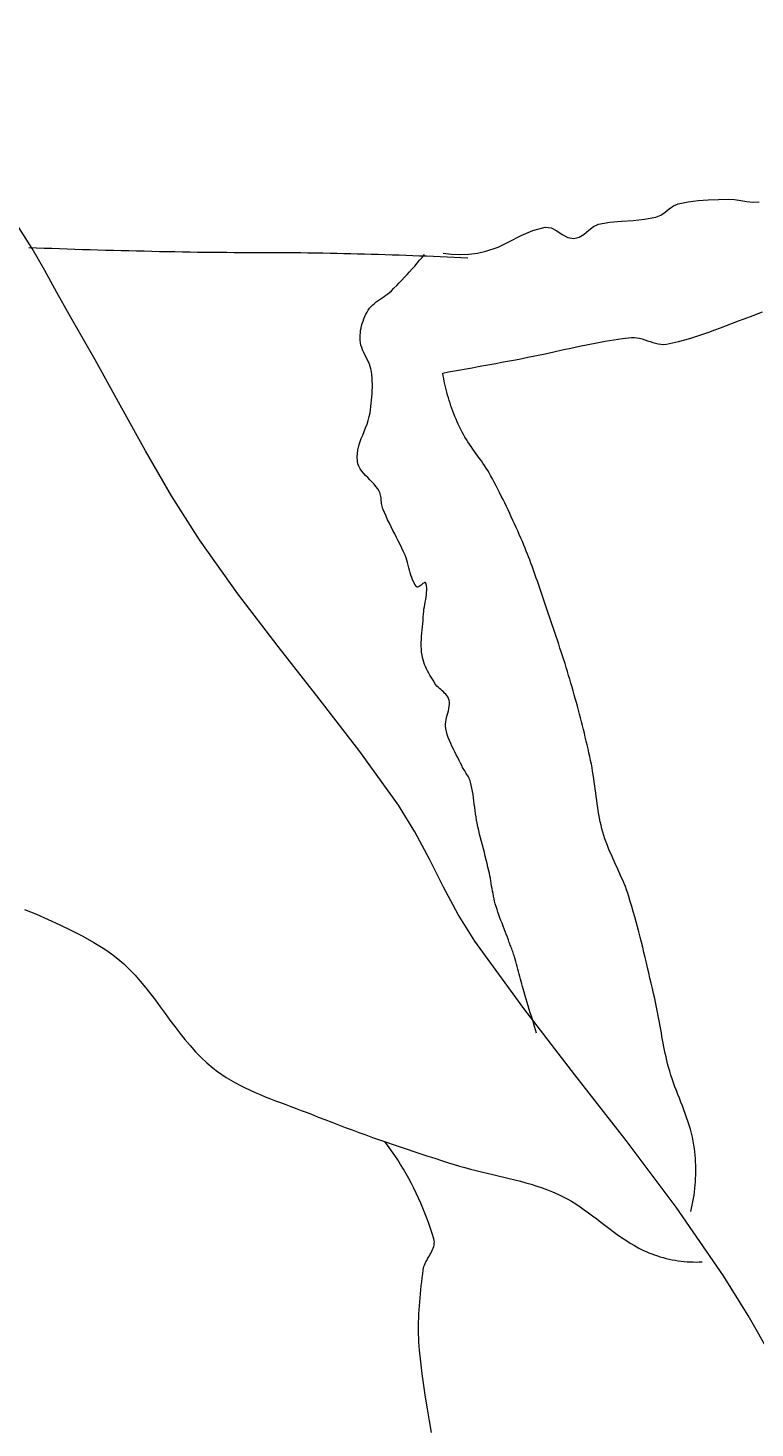
# Model space of a CAD drawing. Units: inches. Extents: x 1441 to 2460, y 1648 to 2683.
# Tile 17 of 35: x 1845 to 1861, y 2091 to 2122. Entities that reach past the tile are written whole.
import ezdxf

# ---------------------------------------------------------------- set-up
doc = ezdxf.new("R2010")
doc.units = ezdxf.units.IN
doc.layers.add('A-ANNO-DIMS', color=2, linetype='Continuous', lineweight=18)
doc.layers.add('A-FURN', color=8, linetype='Continuous', lineweight=15)
doc.styles.get("Standard").update_dxf_attribs({"font": 'arial.ttf'})
doc.dimstyles.get("Standard").update_dxf_attribs({"dimtxt": 0.18, "dimasz": 0.18, "dimexe": 0.18, "dimexo": 0.0625, "dimgap": 0.09, "dimtad": 0, "dimtih": 1, "dimtoh": 1, "dimdec": 4, "dimzin": 0, "dimdsep": 46, "dimtxsty": 'Standard', "dimcen": 0.09, "dimadec": 0, "dimazin": 0, "dimtfac": 1, "dimtdec": 4, "dimtofl": 0, "dimtmove": 0, "dimatfit": 3, "dimfxl": 1, "dimtolj": 1, "dimtzin": 0, "dimarcsym": 0})

# ---------------------------------------------------------------- blocks, each defined once
blk = doc.blocks.new('BED-DOUBLE-PLAN')
for p, q in [((7.216, 72.957), (7.14, 73.155)), ((30.052, 73.35), (29.164, 72.842)), ((4.72, 72.818), (4.732, 72.953)), ((4.732, 72.953), (4.722, 73.087)), ((7.289, 72.758), (7.216, 72.957)), ((29.164, 72.842), (28.298, 72.301)), ((4.668, 72.41), (4.675, 72.546)), ((4.675, 72.546), (4.697, 72.682)), ((4.697, 72.682), (4.72, 72.818)), ((7.337, 72.628), (7.289, 72.758)), ((7.386, 72.498), (7.337, 72.628)), ((4.673, 72.189), (4.668, 72.41)), ((7.436, 72.369), (7.386, 72.498)), ((7.486, 72.239), (7.436, 72.369)), ((7.535, 72.109), (7.486, 72.239)), ((28.298, 72.301), (26.791, 71.264)), ((4.68, 71.967), (4.673, 72.189)), ((4.695, 71.746), (4.68, 71.967)), ((7.583, 71.979), (7.535, 72.109)), ((7.63, 71.848), (7.583, 71.979)), ((4.722, 71.527), (4.695, 71.746)), ((7.675, 71.717), (7.63, 71.848)), ((7.717, 71.585), (7.675, 71.717)), ((25.162, 71.599), (25.076, 71.576)), ((25.25, 71.62), (25.162, 71.599)), ((25.337, 71.638), (25.25, 71.62)), ((25.426, 71.654), (25.337, 71.638)), ((25.498, 71.664), (25.426, 71.654)), ((25.571, 71.673), (25.498, 71.664)), ((25.644, 71.68), (25.571, 71.673)), ((25.717, 71.686), (25.644, 71.68)), ((25.79, 71.691), (25.717, 71.686)), ((25.864, 71.694), (25.79, 71.691)), ((25.938, 71.695), (25.864, 71.694)), ((26.011, 71.695), (25.938, 71.695)), ((26.085, 71.694), (26.011, 71.695)), ((26.159, 71.691), (26.085, 71.694)), ((26.233, 71.687), (26.159, 71.691)), ((26.306, 71.681), (26.233, 71.687)), ((26.379, 71.674), (26.306, 71.681)), ((26.453, 71.665), (26.379, 71.674)), ((26.525, 71.655), (26.453, 71.665)), ((26.598, 71.643), (26.525, 71.655)), ((26.67, 71.63), (26.598, 71.643)), ((26.742, 71.616), (26.67, 71.63)), ((26.814, 71.6), (26.742, 71.616)), ((26.885, 71.583), (26.814, 71.6)), ((27.992, 71.766), (27.99, 71.832)), ((27.99, 71.568), (27.992, 71.634)), ((27.993, 71.7), (27.992, 71.766)), ((27.992, 71.634), (27.993, 71.7)), ((4.765, 71.311), (4.722, 71.527)), ((4.809, 71.206), (4.765, 71.311)), ((7.755, 71.452), (7.717, 71.585)), ((7.79, 71.318), (7.755, 71.452)), ((7.821, 71.184), (7.79, 71.318)), ((24.313, 71.301), (24.228, 71.268)), ((24.397, 71.334), (24.313, 71.301)), ((24.481, 71.366), (24.397, 71.334)), ((24.566, 71.399), (24.481, 71.366)), ((24.65, 71.431), (24.566, 71.399)), ((24.735, 71.463), (24.65, 71.431)), ((24.819, 71.493), (24.735, 71.463)), ((24.904, 71.523), (24.819, 71.493)), ((24.99, 71.55), (24.904, 71.523)), ((25.076, 71.576), (24.99, 71.55)), ((27.953, 71.239), (27.964, 71.304)), ((27.964, 71.304), (27.972, 71.37)), ((27.972, 71.37), (27.98, 71.436)), ((27.98, 71.436), (27.985, 71.502)), ((27.985, 71.502), (27.99, 71.568)), ((4.876, 71.111), (4.809, 71.206)), ((4.95, 71.019), (4.876, 71.111)), ((5.017, 70.924), (4.95, 71.019)), ((7.846, 71.048), (7.821, 71.184)), ((7.852, 70.989), (7.846, 71.048)), ((7.85, 70.93), (7.852, 70.989)), ((23.192, 70.98), (23.116, 70.966)), ((23.267, 70.995), (23.192, 70.98)), ((23.342, 71.01), (23.267, 70.995)), ((23.417, 71.025), (23.342, 71.01)), ((23.492, 71.042), (23.417, 71.025)), ((23.567, 71.059), (23.492, 71.042)), ((23.641, 71.077), (23.567, 71.059)), ((23.715, 71.097), (23.641, 71.077)), ((23.802, 71.121), (23.715, 71.097)), ((23.888, 71.147), (23.802, 71.121)), ((23.974, 71.176), (23.888, 71.147)), ((24.059, 71.205), (23.974, 71.176)), ((24.144, 71.236), (24.059, 71.205)), ((24.228, 71.268), (24.144, 71.236)), ((26.791, 71.264), (25.327, 70.164)), ((27.877, 70.915), (27.895, 70.979)), ((27.895, 70.979), (27.912, 71.044)), ((27.912, 71.044), (27.927, 71.108)), ((27.927, 71.108), (27.941, 71.173)), ((27.941, 71.173), (27.953, 71.239)), ((5.062, 70.82), (5.017, 70.924)), ((5.108, 70.571), (5.062, 70.82)), ((7.772, 70.636), (7.792, 70.694)), ((7.792, 70.694), (7.811, 70.753)), ((7.811, 70.753), (7.828, 70.812)), ((7.828, 70.812), (7.842, 70.871)), ((7.842, 70.871), (7.85, 70.93)), ((21.761, 70.689), (21.648, 70.663)), ((21.874, 70.715), (21.761, 70.689)), ((21.987, 70.741), (21.874, 70.715)), ((22.1, 70.767), (21.987, 70.741)), ((22.212, 70.793), (22.1, 70.767)), ((22.287, 70.81), (22.212, 70.793)), ((22.362, 70.827), (22.287, 70.81)), ((22.437, 70.842), (22.362, 70.827)), ((22.512, 70.857), (22.437, 70.842)), ((22.588, 70.871), (22.512, 70.857)), ((22.663, 70.885), (22.588, 70.871)), ((22.739, 70.899), (22.663, 70.885)), ((22.814, 70.912), (22.739, 70.899)), ((22.89, 70.926), (22.814, 70.912)), ((22.965, 70.939), (22.89, 70.926)), ((23.041, 70.952), (22.965, 70.939)), ((23.116, 70.966), (23.041, 70.952)), ((27.789, 70.666), (27.814, 70.727)), ((27.814, 70.727), (27.836, 70.79)), ((27.836, 70.79), (27.858, 70.852)), ((27.858, 70.852), (27.877, 70.915)), ((5.131, 70.318), (5.108, 70.571)), ((7.703, 70.34), (7.708, 70.399)), ((7.708, 70.399), (7.719, 70.459)), ((7.719, 70.459), (7.734, 70.518)), ((7.734, 70.518), (7.752, 70.577)), ((7.752, 70.577), (7.772, 70.636)), ((20.525, 70.385), (20.413, 70.354)), ((20.636, 70.415), (20.525, 70.385)), ((20.748, 70.444), (20.636, 70.415)), ((20.861, 70.473), (20.748, 70.444)), ((20.973, 70.501), (20.861, 70.473)), ((21.085, 70.529), (20.973, 70.501)), ((21.198, 70.556), (21.085, 70.529)), ((21.31, 70.583), (21.198, 70.556)), ((21.423, 70.61), (21.31, 70.583)), ((21.536, 70.636), (21.423, 70.61)), ((21.648, 70.663), (21.536, 70.636)), ((27.633, 70.347), (27.687, 70.445)), ((27.687, 70.445), (27.736, 70.546)), ((27.736, 70.546), (27.764, 70.606)), ((27.764, 70.606), (27.789, 70.666)), ((5.147, 70.064), (5.131, 70.318)), ((5.17, 69.811), (5.147, 70.064)), ((7.705, 70.28), (7.703, 70.34)), ((7.727, 70.089), (7.705, 70.28)), ((7.754, 69.899), (7.727, 70.089)), ((19.544, 70.06), (19.475, 70.029)), ((19.614, 70.091), (19.544, 70.06)), ((19.684, 70.12), (19.614, 70.091)), ((19.754, 70.148), (19.684, 70.12)), ((19.825, 70.175), (19.754, 70.148)), ((19.897, 70.2), (19.825, 70.175)), ((19.969, 70.223), (19.897, 70.2)), ((20.08, 70.257), (19.969, 70.223)), ((20.191, 70.29), (20.08, 70.257)), ((20.302, 70.323), (20.191, 70.29)), ((20.413, 70.354), (20.302, 70.323)), ((25.327, 70.164), (23.883, 69.037)), ((27.387, 69.97), (27.452, 70.062)), ((27.452, 70.062), (27.515, 70.156)), ((27.515, 70.156), (27.576, 70.251)), ((27.576, 70.251), (27.633, 70.347)), ((5.217, 69.562), (5.17, 69.811)), ((7.784, 69.709), (7.754, 69.899)), ((18.848, 69.753), (18.777, 69.726)), ((18.919, 69.781), (18.848, 69.753)), ((18.989, 69.81), (18.919, 69.781)), ((19.059, 69.841), (18.989, 69.81)), ((19.128, 69.871), (19.059, 69.841)), ((19.197, 69.903), (19.128, 69.871)), ((19.267, 69.935), (19.197, 69.903)), ((19.336, 69.966), (19.267, 69.935)), ((19.405, 69.998), (19.336, 69.966)), ((19.475, 70.029), (19.405, 69.998)), ((27.184, 69.699), (27.253, 69.789)), ((27.253, 69.789), (27.321, 69.879)), ((27.321, 69.879), (27.387, 69.97)), ((5.269, 69.448), (5.217, 69.562)), ((5.347, 69.344), (5.269, 69.448)), ((7.818, 69.519), (7.784, 69.709)), ((7.855, 69.33), (7.818, 69.519)), ((17.301, 69.444), (17.222, 69.431)), ((17.38, 69.456), (17.301, 69.444)), ((17.459, 69.467), (17.38, 69.456)), ((17.538, 69.478), (17.459, 69.467)), ((17.618, 69.488), (17.538, 69.478)), ((17.697, 69.499), (17.618, 69.488)), ((17.777, 69.509), (17.697, 69.499)), ((17.856, 69.52), (17.777, 69.509)), ((17.935, 69.531), (17.856, 69.52)), ((18.014, 69.543), (17.935, 69.531)), ((18.093, 69.555), (18.014, 69.543)), ((18.172, 69.569), (18.093, 69.555)), ((18.25, 69.583), (18.172, 69.569)), ((18.329, 69.599), (18.25, 69.583)), ((18.407, 69.617), (18.329, 69.599)), ((18.484, 69.635), (18.407, 69.617)), ((18.561, 69.656), (18.484, 69.635)), ((18.634, 69.678), (18.561, 69.656)), ((18.706, 69.701), (18.634, 69.678)), ((18.777, 69.726), (18.706, 69.701)), ((26.978, 69.429), (27.046, 69.519)), ((27.046, 69.519), (27.115, 69.609)), ((27.115, 69.609), (27.184, 69.699)), ((5.431, 69.242), (5.347, 69.344)), ((5.5, 69.136), (5.431, 69.242)), ((5.532, 69.019), (5.5, 69.136)), ((7.893, 69.141), (7.855, 69.33)), ((7.934, 68.953), (7.893, 69.141)), ((15.965, 69.142), (15.88, 69.119)), ((16.05, 69.164), (15.965, 69.142)), ((16.134, 69.186), (16.05, 69.164)), ((16.219, 69.207), (16.134, 69.186)), ((16.304, 69.228), (16.219, 69.207)), ((16.389, 69.249), (16.304, 69.228)), ((16.474, 69.27), (16.389, 69.249)), ((16.559, 69.29), (16.474, 69.27)), ((16.644, 69.31), (16.559, 69.29)), ((16.73, 69.33), (16.644, 69.31)), ((16.815, 69.349), (16.73, 69.33)), ((16.901, 69.368), (16.815, 69.349)), ((16.986, 69.387), (16.901, 69.368)), ((17.064, 69.403), (16.986, 69.387)), ((17.143, 69.417), (17.064, 69.403)), ((17.222, 69.431), (17.143, 69.417)), ((26.718, 69.06), (26.78, 69.154)), ((26.78, 69.154), (26.844, 69.246)), ((26.844, 69.246), (26.91, 69.338)), ((26.91, 69.338), (26.978, 69.429)), ((5.44, 68.765), (5.508, 68.888)), ((5.508, 68.888), (5.532, 69.019)), ((7.975, 68.764), (7.934, 68.953)), ((14.946, 68.851), (14.86, 68.824)), ((15.032, 68.877), (14.946, 68.851)), ((15.118, 68.903), (15.032, 68.877)), ((15.204, 68.929), (15.118, 68.903)), ((15.29, 68.954), (15.204, 68.929)), ((15.375, 68.979), (15.29, 68.954)), ((15.459, 69.003), (15.375, 68.979)), ((15.543, 69.026), (15.459, 69.003)), ((15.627, 69.05), (15.543, 69.026)), ((15.711, 69.073), (15.627, 69.05)), ((15.796, 69.096), (15.711, 69.073)), ((15.88, 69.119), (15.796, 69.096)), ((23.883, 69.037), (22.432, 67.918)), ((26.551, 68.769), (26.603, 68.868)), ((26.603, 68.868), (26.659, 68.965)), ((26.659, 68.965), (26.718, 69.06)), ((5.281, 68.391), (5.296, 68.52)), ((5.296, 68.52), (5.359, 68.643)), ((5.359, 68.643), (5.44, 68.765)), ((8.017, 68.576), (7.975, 68.764)), ((8.058, 68.388), (8.017, 68.576)), ((14.006, 68.542), (13.921, 68.513)), ((14.091, 68.571), (14.006, 68.542)), ((14.176, 68.6), (14.091, 68.571)), ((14.262, 68.629), (14.176, 68.6)), ((14.347, 68.657), (14.262, 68.629)), ((14.432, 68.686), (14.347, 68.657)), ((14.518, 68.714), (14.432, 68.686)), ((14.603, 68.742), (14.518, 68.714)), ((14.689, 68.769), (14.603, 68.742)), ((14.774, 68.797), (14.689, 68.769)), ((14.86, 68.824), (14.774, 68.797)), ((26.407, 68.437), (26.453, 68.553)), ((26.453, 68.553), (26.503, 68.668)), ((26.503, 68.668), (26.551, 68.769)), ((5.35, 68.121), (5.281, 68.391)), ((8.098, 68.199), (8.058, 68.388)), ((13.048, 68.217), (12.981, 68.194)), ((13.114, 68.24), (13.048, 68.217)), ((13.181, 68.262), (13.114, 68.24)), ((13.247, 68.285), (13.181, 68.262)), ((13.314, 68.307), (13.247, 68.285)), ((13.381, 68.33), (13.314, 68.307)), ((13.447, 68.352), (13.381, 68.33)), ((13.514, 68.375), (13.447, 68.352)), ((13.58, 68.397), (13.514, 68.375)), ((13.665, 68.426), (13.58, 68.397)), ((13.75, 68.455), (13.665, 68.426)), ((13.836, 68.484), (13.75, 68.455)), ((13.921, 68.513), (13.836, 68.484)), ((26.325, 68.203), (26.365, 68.321)), ((26.365, 68.321), (26.407, 68.437)), ((5.463, 67.863), (5.35, 68.121)), ((8.137, 68.01), (8.098, 68.199)), ((8.174, 67.821), (8.137, 68.01)), ((12.259, 67.921), (12.181, 67.888)), ((12.324, 67.948), (12.259, 67.921)), ((12.389, 67.974), (12.324, 67.948)), ((12.454, 68.001), (12.389, 67.974)), ((12.519, 68.026), (12.454, 68.001)), ((12.585, 68.051), (12.519, 68.026)), ((12.651, 68.076), (12.585, 68.051)), ((12.717, 68.1), (12.651, 68.076)), ((12.783, 68.124), (12.717, 68.1)), ((12.849, 68.148), (12.783, 68.124)), ((12.915, 68.171), (12.849, 68.148)), ((12.981, 68.194), (12.915, 68.171)), ((22.432, 67.918), (20.949, 66.844)), ((21.998, 67.909), (21.944, 67.894)), ((22.073, 67.931), (21.998, 67.909)), ((22.148, 67.953), (22.073, 67.931)), ((22.223, 67.975), (22.148, 67.953)), ((22.297, 67.997), (22.223, 67.975)), ((22.372, 68.019), (22.297, 67.997)), ((22.447, 68.041), (22.372, 68.019)), ((22.521, 68.063), (22.447, 68.041)), ((22.596, 68.086), (22.521, 68.063)), ((22.671, 68.108), (22.596, 68.086)), ((22.745, 68.131), (22.671, 68.108)), ((22.82, 68.154), (22.745, 68.131)), ((22.894, 68.176), (22.82, 68.154)), ((22.969, 68.199), (22.894, 68.176)), ((26.219, 67.844), (26.252, 67.965)), ((26.252, 67.965), (26.287, 68.084)), ((26.287, 68.084), (26.325, 68.203)), ((5.593, 67.609), (5.463, 67.863)), ((5.717, 67.354), (5.593, 67.609)), ((8.198, 67.692), (8.174, 67.821)), ((8.222, 67.563), (8.198, 67.692)), ((11.562, 67.611), (11.486, 67.574)), ((11.639, 67.646), (11.562, 67.611)), ((11.716, 67.682), (11.639, 67.646)), ((11.793, 67.717), (11.716, 67.682)), ((11.87, 67.752), (11.793, 67.717)), ((11.948, 67.786), (11.87, 67.752)), ((12.025, 67.82), (11.948, 67.786)), ((12.103, 67.854), (12.025, 67.82)), ((12.181, 67.888), (12.103, 67.854)), ((20.979, 67.602), (20.95, 67.591)), ((21.007, 67.612), (20.979, 67.602)), ((21.036, 67.623), (21.007, 67.612)), ((21.064, 67.634), (21.036, 67.623)), ((21.092, 67.645), (21.064, 67.634)), ((21.12, 67.655), (21.092, 67.645)), ((21.149, 67.666), (21.12, 67.655)), ((21.177, 67.676), (21.149, 67.666)), ((21.206, 67.686), (21.177, 67.676)), ((21.234, 67.696), (21.206, 67.686)), ((21.263, 67.705), (21.234, 67.696)), ((21.292, 67.714), (21.263, 67.705)), ((21.346, 67.73), (21.292, 67.714)), ((21.4, 67.746), (21.346, 67.73)), ((21.454, 67.761), (21.4, 67.746)), ((21.509, 67.776), (21.454, 67.761)), ((21.563, 67.791), (21.509, 67.776)), ((21.617, 67.806), (21.563, 67.791)), ((21.672, 67.82), (21.617, 67.806)), ((21.726, 67.835), (21.672, 67.82)), ((21.781, 67.849), (21.726, 67.835)), ((21.835, 67.864), (21.781, 67.849)), ((21.89, 67.879), (21.835, 67.864)), ((21.944, 67.894), (21.89, 67.879)), ((26.127, 67.481), (26.156, 67.602)), ((26.156, 67.602), (26.187, 67.724)), ((26.187, 67.724), (26.219, 67.844)), ((5.81, 67.088), (5.717, 67.354)), ((8.246, 67.434), (8.222, 67.563)), ((8.27, 67.304), (8.246, 67.434)), ((8.294, 67.175), (8.27, 67.304)), ((10.955, 67.31), (10.88, 67.271)), ((11.03, 67.349), (10.955, 67.31)), ((11.105, 67.388), (11.03, 67.349)), ((11.181, 67.426), (11.105, 67.388)), ((11.257, 67.464), (11.181, 67.426)), ((11.333, 67.501), (11.257, 67.464)), ((11.409, 67.538), (11.333, 67.501)), ((11.486, 67.574), (11.409, 67.538)), ((20.129, 67.295), (20.074, 67.28)), ((20.191, 67.313), (20.129, 67.295)), ((20.253, 67.333), (20.191, 67.313)), ((20.315, 67.353), (20.253, 67.333)), ((20.376, 67.375), (20.315, 67.353)), ((20.437, 67.397), (20.376, 67.375)), ((20.498, 67.419), (20.437, 67.397)), ((20.558, 67.442), (20.498, 67.419)), ((20.619, 67.466), (20.558, 67.442)), ((20.679, 67.489), (20.619, 67.466)), ((20.74, 67.513), (20.679, 67.489)), ((20.8, 67.536), (20.74, 67.513)), ((20.861, 67.559), (20.8, 67.536)), ((20.922, 67.581), (20.861, 67.559)), ((20.95, 67.591), (20.922, 67.581)), ((26.069, 67.237), (26.098, 67.359)), ((26.098, 67.359), (26.127, 67.481)), ((5.849, 66.904), (5.81, 67.088)), ((8.318, 67.046), (8.294, 67.175)), ((8.341, 66.917), (8.318, 67.046)), ((10.409, 66.988), (10.357, 66.951)), ((10.461, 67.024), (10.409, 66.988)), ((10.514, 67.059), (10.461, 67.024)), ((10.567, 67.094), (10.514, 67.059)), ((10.621, 67.127), (10.567, 67.094)), ((10.675, 67.159), (10.621, 67.127)), ((10.731, 67.191), (10.675, 67.159)), ((10.805, 67.231), (10.731, 67.191)), ((10.88, 67.271), (10.805, 67.231)), ((18.764, 66.991), (18.683, 66.971)), ((18.843, 67.012), (18.764, 66.991)), ((18.923, 67.033), (18.843, 67.012)), ((19.003, 67.054), (18.923, 67.033)), ((19.083, 67.074), (19.003, 67.054)), ((19.163, 67.095), (19.083, 67.074)), ((19.243, 67.115), (19.163, 67.095)), ((19.324, 67.134), (19.243, 67.115)), ((19.404, 67.153), (19.324, 67.134)), ((19.46, 67.165), (19.404, 67.153)), ((19.515, 67.176), (19.46, 67.165)), ((19.571, 67.186), (19.515, 67.176)), ((19.628, 67.196), (19.571, 67.186)), ((19.684, 67.205), (19.628, 67.196)), ((19.74, 67.214), (19.684, 67.205)), ((19.796, 67.224), (19.74, 67.214)), ((19.852, 67.234), (19.796, 67.224)), ((19.908, 67.244), (19.852, 67.234)), ((19.964, 67.255), (19.908, 67.244)), ((20.019, 67.267), (19.964, 67.255)), ((20.074, 67.28), (20.019, 67.267)), ((25.982, 66.871), (26.012, 66.993)), ((26.012, 66.993), (26.041, 67.115)), ((26.041, 67.115), (26.069, 67.237)), ((5.873, 66.715), (5.849, 66.904)), ((5.881, 66.525), (5.873, 66.715)), ((5.946, 66.541), (5.953, 66.692)), ((8.365, 66.787), (8.341, 66.917)), ((8.388, 66.658), (8.365, 66.787)), ((9.992, 66.695), (9.939, 66.661)), ((10.045, 66.731), (9.992, 66.695)), ((10.097, 66.767), (10.045, 66.731)), ((10.149, 66.803), (10.097, 66.767)), ((10.201, 66.84), (10.149, 66.803)), ((10.253, 66.877), (10.201, 66.84)), ((10.305, 66.914), (10.253, 66.877)), ((10.357, 66.951), (10.305, 66.914)), ((17.32, 66.689), (17.294, 66.673)), ((17.347, 66.704), (17.32, 66.689)), ((17.374, 66.718), (17.347, 66.704)), ((17.402, 66.73), (17.374, 66.718)), ((17.43, 66.741), (17.402, 66.73)), ((17.459, 66.75), (17.43, 66.741)), ((17.527, 66.767), (17.459, 66.75)), ((17.596, 66.782), (17.527, 66.767)), ((17.665, 66.794), (17.596, 66.782)), ((17.734, 66.806), (17.665, 66.794)), ((17.804, 66.816), (17.734, 66.806)), ((17.874, 66.825), (17.804, 66.816)), ((17.944, 66.834), (17.874, 66.825)), ((18.014, 66.843), (17.944, 66.834)), ((18.084, 66.851), (18.014, 66.843)), ((18.154, 66.861), (18.084, 66.851)), ((18.223, 66.871), (18.154, 66.861)), ((18.293, 66.883), (18.223, 66.871)), ((18.362, 66.897), (18.293, 66.883)), ((18.443, 66.914), (18.362, 66.897)), ((18.523, 66.932), (18.443, 66.914)), ((18.603, 66.951), (18.523, 66.932)), ((18.683, 66.971), (18.603, 66.951)), ((20.949, 66.844), (20.369, 66.483)), ((25.92, 66.629), (25.952, 66.75)), ((25.952, 66.75), (25.982, 66.871)), ((5.874, 66.335), (5.881, 66.525)), ((5.932, 66.239), (5.939, 66.39)), ((5.939, 66.39), (5.946, 66.541)), ((8.412, 66.529), (8.388, 66.658)), ((8.435, 66.399), (8.412, 66.529)), ((8.458, 66.27), (8.435, 66.399)), ((9.378, 66.386), (9.32, 66.364)), ((9.436, 66.408), (9.378, 66.386)), ((9.493, 66.432), (9.436, 66.408)), ((9.55, 66.456), (9.493, 66.432)), ((9.607, 66.481), (9.55, 66.456)), ((9.663, 66.507), (9.607, 66.481)), ((9.72, 66.535), (9.663, 66.507)), ((9.776, 66.564), (9.72, 66.535)), ((9.831, 66.595), (9.776, 66.564)), ((9.886, 66.627), (9.831, 66.595)), ((9.939, 66.661), (9.886, 66.627)), ((16.734, 66.375), (16.672, 66.344)), ((16.797, 66.407), (16.734, 66.375)), ((16.859, 66.439), (16.797, 66.407)), ((16.921, 66.471), (16.859, 66.439)), ((16.983, 66.503), (16.921, 66.471)), ((17.045, 66.534), (16.983, 66.503)), ((17.108, 66.564), (17.045, 66.534)), ((17.136, 66.577), (17.108, 66.564)), ((17.163, 66.592), (17.136, 66.577)), ((17.189, 66.608), (17.163, 66.592)), ((17.215, 66.624), (17.189, 66.608)), ((17.241, 66.64), (17.215, 66.624)), ((17.268, 66.657), (17.241, 66.64)), ((17.294, 66.673), (17.268, 66.657)), ((20.369, 66.483), (19.765, 66.161)), ((25.815, 66.269), (25.852, 66.388)), ((25.852, 66.388), (25.887, 66.508)), ((25.887, 66.508), (25.92, 66.629)), ((5.851, 66.148), (5.874, 66.335)), ((5.92, 65.936), (5.926, 66.088)), ((5.926, 66.088), (5.932, 66.239)), ((8.481, 66.141), (8.458, 66.27)), ((8.542, 66.151), (8.481, 66.141)), ((8.603, 66.163), (8.542, 66.151)), ((8.664, 66.175), (8.603, 66.163)), ((8.725, 66.188), (8.664, 66.175)), ((8.785, 66.202), (8.725, 66.188)), ((8.845, 66.216), (8.785, 66.202)), ((8.905, 66.232), (8.845, 66.216)), ((8.965, 66.248), (8.905, 66.232)), ((9.025, 66.266), (8.965, 66.248)), ((9.085, 66.284), (9.025, 66.266)), ((9.144, 66.303), (9.085, 66.284)), ((9.203, 66.322), (9.144, 66.303)), ((9.262, 66.342), (9.203, 66.322)), ((9.32, 66.364), (9.262, 66.342)), ((15.405, 66.068), (15.379, 66.04)), ((15.43, 66.097), (15.405, 66.068)), ((15.455, 66.127), (15.43, 66.097)), ((15.481, 66.156), (15.455, 66.127)), ((15.506, 66.183), (15.481, 66.156)), ((15.533, 66.209), (15.506, 66.183)), ((15.561, 66.233), (15.533, 66.209)), ((15.591, 66.253), (15.561, 66.233)), ((15.623, 66.268), (15.591, 66.253)), ((15.658, 66.28), (15.623, 66.268)), ((15.705, 66.287), (15.658, 66.28)), ((15.752, 66.289), (15.705, 66.287)), ((15.8, 66.285), (15.752, 66.289)), ((15.848, 66.277), (15.8, 66.285)), ((15.896, 66.266), (15.848, 66.277)), ((15.945, 66.253), (15.896, 66.266)), ((15.993, 66.239), (15.945, 66.253)), ((16.042, 66.226), (15.993, 66.239)), ((16.09, 66.215), (16.042, 66.226)), ((16.138, 66.206), (16.09, 66.215)), ((16.186, 66.2), (16.138, 66.206)), ((16.234, 66.2), (16.186, 66.2)), ((16.282, 66.206), (16.234, 66.2)), ((16.349, 66.221), (16.282, 66.206)), ((16.415, 66.24), (16.349, 66.221)), ((16.48, 66.263), (16.415, 66.24)), ((16.545, 66.288), (16.48, 66.263)), ((16.609, 66.315), (16.545, 66.288)), ((16.672, 66.344), (16.609, 66.315)), ((19.765, 66.161), (19.153, 65.853)), ((25.716, 65.966), (25.765, 66.117)), ((25.765, 66.117), (25.815, 66.269)), ((5.908, 65.634), (5.913, 65.785)), ((5.913, 65.785), (5.92, 65.936)), ((13.081, 65.766), (13.078, 65.756)), ((13.078, 65.756), (13.081, 65.742)), ((13.093, 65.773), (13.081, 65.766)), ((13.144, 65.784), (13.093, 65.773)), ((13.195, 65.789), (13.144, 65.784)), ((13.247, 65.791), (13.195, 65.789)), ((13.298, 65.788), (13.247, 65.791)), ((13.35, 65.783), (13.298, 65.788)), ((13.403, 65.776), (13.35, 65.783)), ((13.455, 65.767), (13.403, 65.776)), ((13.508, 65.757), (13.455, 65.767)), ((13.56, 65.747), (13.508, 65.757)), ((14.924, 65.764), (14.876, 65.744)), ((14.972, 65.786), (14.924, 65.764)), ((15.019, 65.81), (14.972, 65.786)), ((15.066, 65.835), (15.019, 65.81)), ((15.112, 65.861), (15.066, 65.835)), ((15.157, 65.887), (15.112, 65.861)), ((15.202, 65.914), (15.157, 65.887)), ((15.247, 65.942), (15.202, 65.914)), ((15.292, 65.969), (15.247, 65.942)), ((15.323, 65.99), (15.292, 65.969)), ((15.351, 66.014), (15.323, 65.99)), ((15.379, 66.04), (15.351, 66.014)), ((19.153, 65.853), (18.549, 65.531)), ((25.616, 65.662), (25.666, 65.814)), ((25.666, 65.814), (25.716, 65.966)), ((27.033, 65.794), (26.921, 65.751)), ((27.145, 65.835), (27.033, 65.794)), ((27.257, 65.874), (27.145, 65.835)), ((27.37, 65.911), (27.257, 65.874)), ((27.484, 65.946), (27.37, 65.911)), ((27.519, 65.953), (27.484, 65.946)), ((27.553, 65.957), (27.519, 65.953)), ((27.587, 65.955), (27.553, 65.957)), ((27.62, 65.951), (27.587, 65.955)), ((27.654, 65.942), (27.62, 65.951)), ((27.688, 65.931), (27.654, 65.942)), ((27.721, 65.918), (27.688, 65.931)), ((27.755, 65.902), (27.721, 65.918)), ((27.788, 65.885), (27.755, 65.902)), ((27.822, 65.867), (27.788, 65.885)), ((27.855, 65.847), (27.822, 65.867)), ((27.889, 65.828), (27.855, 65.847)), ((27.923, 65.809), (27.889, 65.828)), ((27.957, 65.79), (27.923, 65.809)), ((27.991, 65.772), (27.957, 65.79)), ((28.025, 65.756), (27.991, 65.772)), ((28.06, 65.741), (28.025, 65.756)), ((30.96, 65.765), (30.702, 65.727)), ((31.218, 65.805), (30.96, 65.765)), ((31.475, 65.847), (31.218, 65.805)), ((31.732, 65.891), (31.475, 65.847)), ((5.943, 65.687), (5.879, 65.74)), ((5.896, 65.332), (5.902, 65.483)), ((5.902, 65.483), (5.908, 65.634)), ((6.006, 65.633), (5.943, 65.687)), ((6.07, 65.579), (6.006, 65.633)), ((6.133, 65.525), (6.07, 65.579)), ((6.195, 65.47), (6.133, 65.525)), ((6.257, 65.414), (6.195, 65.47)), ((12.972, 65.46), (12.919, 65.442)), ((13.024, 65.48), (12.972, 65.46)), ((13.075, 65.503), (13.024, 65.48)), ((13.123, 65.53), (13.075, 65.503)), ((13.081, 65.742), (13.09, 65.726)), ((13.09, 65.726), (13.103, 65.707)), ((13.103, 65.707), (13.118, 65.687)), ((13.118, 65.687), (13.135, 65.667)), ((13.169, 65.562), (13.123, 65.53)), ((13.135, 65.667), (13.151, 65.646)), ((13.151, 65.646), (13.164, 65.626)), ((13.164, 65.626), (13.175, 65.606)), ((13.179, 65.574), (13.169, 65.562)), ((13.175, 65.606), (13.18, 65.589)), ((13.18, 65.589), (13.179, 65.574)), ((13.613, 65.738), (13.56, 65.747)), ((13.665, 65.729), (13.613, 65.738)), ((13.718, 65.723), (13.665, 65.729)), ((13.77, 65.718), (13.718, 65.723)), ((13.84, 65.714), (13.77, 65.718)), ((13.91, 65.708), (13.84, 65.714)), ((13.98, 65.701), (13.91, 65.708)), ((14.05, 65.694), (13.98, 65.701)), ((14.12, 65.688), (14.05, 65.694)), ((14.19, 65.681), (14.12, 65.688)), ((14.26, 65.676), (14.19, 65.681)), ((14.33, 65.672), (14.26, 65.676)), ((14.399, 65.669), (14.33, 65.672)), ((14.469, 65.669), (14.399, 65.669)), ((14.539, 65.672), (14.469, 65.669)), ((14.608, 65.678), (14.539, 65.672)), ((14.677, 65.687), (14.608, 65.678)), ((14.728, 65.697), (14.677, 65.687)), ((14.778, 65.71), (14.728, 65.697)), ((14.828, 65.726), (14.778, 65.71)), ((14.876, 65.744), (14.828, 65.726)), ((18.549, 65.531), (17.968, 65.172)), ((25.515, 65.359), (25.566, 65.51)), ((25.566, 65.51), (25.616, 65.662)), ((26.269, 65.452), (26.163, 65.395)), ((26.375, 65.506), (26.269, 65.452)), ((26.483, 65.559), (26.375, 65.506)), ((26.591, 65.61), (26.483, 65.559)), ((26.7, 65.659), (26.591, 65.61)), ((26.81, 65.706), (26.7, 65.659)), ((26.921, 65.751), (26.81, 65.706)), ((28.094, 65.729), (28.06, 65.741)), ((28.13, 65.72), (28.094, 65.729)), ((28.165, 65.713), (28.13, 65.72)), ((28.253, 65.702), (28.165, 65.713)), ((28.34, 65.691), (28.253, 65.702)), ((28.428, 65.681), (28.34, 65.691)), ((28.516, 65.67), (28.428, 65.681)), ((28.604, 65.661), (28.516, 65.67)), ((28.692, 65.652), (28.604, 65.661)), ((28.78, 65.643), (28.692, 65.652)), ((28.869, 65.635), (28.78, 65.643)), ((28.957, 65.628), (28.869, 65.635)), ((29.045, 65.622), (28.957, 65.628)), ((29.133, 65.617), (29.045, 65.622)), ((29.222, 65.613), (29.133, 65.617)), ((29.31, 65.611), (29.222, 65.613)), ((29.398, 65.609), (29.31, 65.611)), ((29.487, 65.609), (29.398, 65.609)), ((29.575, 65.61), (29.487, 65.609)), ((29.663, 65.613), (29.575, 65.61)), ((29.751, 65.618), (29.663, 65.613)), ((29.839, 65.624), (29.751, 65.618)), ((29.927, 65.632), (29.839, 65.624)), ((30.186, 65.66), (29.927, 65.632)), ((30.444, 65.692), (30.186, 65.66)), ((30.702, 65.727), (30.444, 65.692)), ((5.886, 65.029), (5.891, 65.181)), ((5.891, 65.181), (5.896, 65.332)), ((6.319, 65.358), (6.257, 65.414)), ((6.38, 65.302), (6.319, 65.358)), ((6.44, 65.245), (6.38, 65.302)), ((6.501, 65.188), (6.44, 65.245)), ((6.56, 65.13), (6.501, 65.188)), ((12.168, 65.166), (12.09, 65.127)), ((12.246, 65.204), (12.168, 65.166)), ((12.324, 65.242), (12.246, 65.204)), ((12.403, 65.279), (12.324, 65.242)), ((12.482, 65.314), (12.403, 65.279)), ((12.535, 65.335), (12.482, 65.314)), ((12.588, 65.353), (12.535, 65.335)), ((12.643, 65.369), (12.588, 65.353)), ((12.698, 65.384), (12.643, 65.369)), ((12.754, 65.398), (12.698, 65.384)), ((12.809, 65.412), (12.754, 65.398)), ((12.864, 65.426), (12.809, 65.412)), ((12.919, 65.442), (12.864, 65.426)), ((17.968, 65.172), (16.787, 64.32)), ((25.413, 65.056), (25.464, 65.207)), ((25.464, 65.207), (25.515, 65.359)), ((25.752, 65.152), (25.652, 65.087)), ((25.853, 65.215), (25.752, 65.152)), ((25.955, 65.277), (25.853, 65.215)), ((26.059, 65.337), (25.955, 65.277)), ((26.163, 65.395), (26.059, 65.337)), ((5.876, 64.727), (5.881, 64.878)), ((5.881, 64.878), (5.886, 65.029)), ((6.619, 65.071), (6.56, 65.13)), ((6.678, 65.013), (6.619, 65.071)), ((6.713, 64.975), (6.678, 65.013)), ((6.745, 64.936), (6.713, 64.975)), ((6.776, 64.895), (6.745, 64.936)), ((6.805, 64.853), (6.776, 64.895)), ((6.834, 64.81), (6.805, 64.853)), ((11.544, 64.86), (11.463, 64.827)), ((11.623, 64.896), (11.544, 64.86)), ((11.702, 64.932), (11.623, 64.896)), ((11.78, 64.97), (11.702, 64.932)), ((11.858, 65.008), (11.78, 64.97)), ((11.935, 65.048), (11.858, 65.008)), ((12.013, 65.087), (11.935, 65.048)), ((12.09, 65.127), (12.013, 65.087)), ((25.308, 64.754), (25.361, 64.905)), ((25.456, 64.951), (25.36, 64.881)), ((25.361, 64.905), (25.413, 65.056)), ((25.553, 65.02), (25.456, 64.951)), ((25.652, 65.087), (25.553, 65.02)), ((5.868, 64.425), (5.872, 64.576)), ((5.872, 64.576), (5.876, 64.727)), ((6.863, 64.767), (6.834, 64.81)), ((6.892, 64.724), (6.863, 64.767)), ((6.922, 64.683), (6.892, 64.724)), ((6.953, 64.643), (6.922, 64.683)), ((6.985, 64.605), (6.953, 64.643)), ((7.021, 64.569), (6.985, 64.605)), ((7.058, 64.536), (7.021, 64.569)), ((7.099, 64.507), (7.058, 64.536)), ((8.286, 64.53), (8.234, 64.508)), ((8.339, 64.55), (8.286, 64.53)), ((8.393, 64.565), (8.339, 64.55)), ((8.448, 64.576), (8.393, 64.565)), ((8.518, 64.584), (8.448, 64.576)), ((8.587, 64.59), (8.518, 64.584)), ((8.657, 64.594), (8.587, 64.59)), ((8.727, 64.596), (8.657, 64.594)), ((8.797, 64.596), (8.727, 64.596)), ((8.867, 64.594), (8.797, 64.596)), ((8.937, 64.591), (8.867, 64.594)), ((9.007, 64.586), (8.937, 64.591)), ((9.077, 64.58), (9.007, 64.586)), ((9.147, 64.573), (9.077, 64.58)), ((9.217, 64.564), (9.147, 64.573)), ((9.286, 64.555), (9.217, 64.564)), ((9.355, 64.545), (9.286, 64.555)), ((9.438, 64.528), (9.355, 64.545)), ((9.52, 64.506), (9.438, 64.528)), ((10.824, 64.541), (10.777, 64.494)), ((10.871, 64.588), (10.824, 64.541)), ((10.919, 64.633), (10.871, 64.588)), ((10.969, 64.676), (10.919, 64.633)), ((11.02, 64.714), (10.969, 64.676)), ((11.074, 64.746), (11.02, 64.714)), ((11.102, 64.759), (11.074, 64.746)), ((11.13, 64.769), (11.102, 64.759)), ((11.16, 64.777), (11.13, 64.769)), ((11.19, 64.782), (11.16, 64.777)), ((11.22, 64.787), (11.19, 64.782)), ((11.251, 64.79), (11.22, 64.787)), ((11.282, 64.793), (11.251, 64.79)), ((11.313, 64.796), (11.282, 64.793)), ((11.344, 64.799), (11.313, 64.796)), ((11.375, 64.803), (11.344, 64.799)), ((11.405, 64.809), (11.375, 64.803)), ((11.435, 64.817), (11.405, 64.809)), ((11.463, 64.827), (11.435, 64.817)), ((25.202, 64.453), (25.256, 64.603)), ((25.256, 64.603), (25.308, 64.754)), ((5.86, 64.122), (5.863, 64.273)), ((5.863, 64.273), (5.868, 64.425)), ((7.145, 64.48), (7.099, 64.507)), ((7.192, 64.455), (7.145, 64.48)), ((7.24, 64.432), (7.192, 64.455)), ((7.289, 64.411), (7.24, 64.432)), ((7.34, 64.392), (7.289, 64.411)), ((7.391, 64.375), (7.34, 64.392)), ((7.443, 64.361), (7.391, 64.375)), ((7.496, 64.349), (7.443, 64.361)), ((7.549, 64.339), (7.496, 64.349)), ((7.602, 64.333), (7.549, 64.339)), ((7.655, 64.328), (7.602, 64.333)), ((7.708, 64.327), (7.655, 64.328)), ((7.761, 64.328), (7.708, 64.327)), ((7.817, 64.334), (7.761, 64.328)), ((7.871, 64.346), (7.817, 64.334)), ((7.924, 64.363), (7.871, 64.346)), ((7.976, 64.383), (7.924, 64.363)), ((8.028, 64.406), (7.976, 64.383)), ((8.08, 64.431), (8.028, 64.406)), ((8.131, 64.457), (8.08, 64.431)), ((8.183, 64.483), (8.131, 64.457)), ((8.234, 64.508), (8.183, 64.483)), ((9.601, 64.479), (9.52, 64.506)), ((9.682, 64.449), (9.601, 64.479)), ((9.762, 64.417), (9.682, 64.449)), ((9.842, 64.385), (9.762, 64.417)), ((9.922, 64.354), (9.842, 64.385)), ((10.003, 64.325), (9.922, 64.354)), ((10.083, 64.301), (10.003, 64.325)), ((10.164, 64.281), (10.083, 64.301)), ((10.246, 64.268), (10.164, 64.281)), ((10.328, 64.264), (10.246, 64.268)), ((10.411, 64.268), (10.328, 64.264)), ((10.471, 64.28), (10.411, 64.268)), ((10.528, 64.301), (10.471, 64.28)), ((10.582, 64.33), (10.528, 64.301)), ((10.633, 64.365), (10.582, 64.33)), ((10.682, 64.405), (10.633, 64.365)), ((10.73, 64.448), (10.682, 64.405)), ((10.777, 64.494), (10.73, 64.448)), ((16.787, 64.32), (15.632, 63.429)), ((25.093, 64.152), (25.148, 64.303)), ((25.148, 64.303), (25.202, 64.453)), ((5.852, 63.82), (5.856, 63.971)), ((5.856, 63.971), (5.86, 64.122)), ((24.982, 63.853), (25.038, 64.003)), ((25.038, 64.003), (25.093, 64.152)), ((5.846, 63.507), (5.849, 63.668)), ((5.849, 63.668), (5.852, 63.82)), ((24.868, 63.555), (24.925, 63.704)), ((24.925, 63.704), (24.982, 63.853)), ((5.841, 63.183), (5.843, 63.345)), ((5.843, 63.345), (5.846, 63.507)), ((15.632, 63.429), (14.485, 62.528)), ((24.751, 63.258), (24.81, 63.406)), ((24.81, 63.406), (24.868, 63.555)), ((5.838, 62.86), (5.839, 63.021)), ((5.839, 63.021), (5.841, 63.183)), ((24.621, 62.923), (24.664, 63.035)), ((24.664, 63.035), (24.707, 63.147)), ((24.707, 63.147), (24.751, 63.258)), ((5.836, 62.536), (5.837, 62.698)), ((5.837, 62.698), (5.838, 62.86)), ((24.495, 62.584), (24.537, 62.697)), ((24.537, 62.697), (24.579, 62.81)), ((24.579, 62.81), (24.621, 62.923)), ((5.835, 62.374), (5.836, 62.536)), ((5.835, 62.213), (5.835, 62.374)), ((14.485, 62.528), (13.327, 61.643)), ((24.409, 62.359), (24.452, 62.471)), ((24.452, 62.471), (24.495, 62.584)), ((5.834, 62.051), (5.835, 62.213)), ((24.271, 62.025), (24.319, 62.135)), ((24.319, 62.135), (24.364, 62.247)), ((24.364, 62.247), (24.409, 62.359)), ((5.833, 61.727), (5.834, 61.889)), ((5.834, 61.889), (5.834, 62.051)), ((24.119, 61.701), (24.172, 61.808)), ((24.172, 61.808), (24.223, 61.916)), ((24.223, 61.916), (24.271, 62.025)), ((5.832, 61.404), (5.833, 61.565)), ((5.833, 61.565), (5.833, 61.727)), ((13.327, 61.643), (12.139, 60.8)), ((23.943, 61.391), (24.004, 61.492)), ((24.004, 61.492), (24.063, 61.596)), ((24.063, 61.596), (24.119, 61.701)), ((5.83, 61.08), (5.831, 61.242)), ((5.831, 61.242), (5.832, 61.404)), ((23.737, 61.1), (23.809, 61.195)), ((23.809, 61.195), (23.878, 61.292)), ((23.878, 61.292), (23.943, 61.391)), ((5.826, 60.757), (5.828, 60.918)), ((5.828, 60.918), (5.83, 61.08)), ((23.502, 60.838), (23.623, 60.966)), ((23.623, 60.966), (23.737, 61.1)), ((5.821, 60.433), (5.824, 60.595)), ((5.824, 60.595), (5.826, 60.757)), ((12.139, 60.8), (11.176, 60.189)), ((23.108, 60.482), (23.244, 60.596)), ((23.244, 60.596), (23.376, 60.715)), ((23.376, 60.715), (23.502, 60.838)), ((5.815, 60.095), (5.818, 60.264)), ((5.818, 60.264), (5.821, 60.433)), ((22.683, 60.154), (22.826, 60.262)), ((22.826, 60.262), (22.968, 60.371)), ((22.968, 60.371), (23.108, 60.482)), ((5.807, 59.757), (5.811, 59.926)), ((5.811, 59.926), (5.815, 60.095)), ((11.176, 60.189), (10.189, 59.615)), ((22.249, 59.835), (22.393, 59.942)), ((22.393, 59.942), (22.538, 60.048)), ((22.538, 60.048), (22.683, 60.154)), ((5.803, 59.588), (5.807, 59.757)), ((10.189, 59.615), (9.189, 59.061)), ((21.83, 59.504), (21.967, 59.617)), ((21.967, 59.617), (22.107, 59.727)), ((22.107, 59.727), (22.249, 59.835)), ((5.795, 59.25), (5.799, 59.419)), ((5.799, 59.419), (5.803, 59.588)), ((21.571, 59.267), (21.698, 59.388)), ((21.698, 59.388), (21.83, 59.504)), ((5.786, 58.912), (5.791, 59.081)), ((5.791, 59.081), (5.795, 59.25)), ((9.189, 59.061), (8.189, 58.51)), ((21.227, 58.872), (21.335, 59.01)), ((21.335, 59.01), (21.449, 59.141)), ((21.449, 59.141), (21.571, 59.267)), ((5.777, 58.575), (5.782, 58.743)), ((5.782, 58.743), (5.786, 58.912)), ((20.982, 58.486), (21.129, 58.727)), ((21.129, 58.727), (21.227, 58.872)), ((5.767, 58.237), (5.772, 58.406)), ((5.772, 58.406), (5.777, 58.575)), ((8.189, 58.51), (7.197, 57.943)), ((20.844, 58.24), (20.982, 58.486)), ((5.761, 58.068), (5.767, 58.237)), ((20.714, 57.991), (20.844, 58.24)), ((5.75, 57.73), (5.756, 57.899)), ((5.756, 57.899), (5.761, 58.068)), ((7.197, 57.943), (6.716, 57.672)), ((20.59, 57.739), (20.714, 57.991)), ((5.738, 57.392), (5.744, 57.561)), ((5.744, 57.561), (5.75, 57.73)), ((6.716, 57.672), (6.229, 57.407)), ((20.361, 57.224), (20.473, 57.483)), ((20.473, 57.483), (20.59, 57.739)), ((5.726, 57.054), (5.732, 57.223)), ((5.732, 57.223), (5.738, 57.392)), ((6.229, 57.407), (5.748, 57.134)), ((20.254, 56.963), (20.361, 57.224)), ((5.748, 57.134), (5.285, 56.837))]:
    blk.add_line(p, q)
blk = doc.blocks.new('*D67')
at = {"layer": 'A-ANNO-DIMS', "color": 0, "lineweight": -2, "transparency": 16777216}
for p, q in [((1889.448, 2298.695), (1916.216, 2298.695)), ((1916.036, 2298.515), (1916.036, 2055.938)), ((1916.036, 1812.997), (1916.036, 2055.574)), ((1758.224, 1812.817), (1916.216, 1812.817))]:
    blk.add_line(p, q, dxfattribs=at)
at = {"layer": 'A-ANNO-DIMS', "color": 0, "transparency": 16777216}
for points in [[(1916.006, 2298.515), (1916.066, 2298.515), (1916.036, 2298.695)], [(1916.006, 1812.997), (1916.066, 1812.997), (1916.036, 1812.817)]]:
    blk.add_solid(points, dxfattribs=at)
at = {"layer": 'Defpoints', "color": 0, "transparency": 16777216}
for p in [(1889.386, 2298.695), (1916.036, 2298.695), (1758.161, 1812.817)]:
    blk.add_point(p, dxfattribs=at)
at = {"layer": 'A-ANNO-DIMS', "color": 0, "transparency": 16777216, "insert": (1916.036, 2055.756), "char_height": 0.18, "attachment_point": 5}
blk.add_mtext('\\A1;485.9', dxfattribs=at)

msp = doc.modelspace()

# ---------------------------------------------------------------- block references
at = {"layer": 'A-FURN', "rotation": 270}
msp.add_blockref('BED-DOUBLE-PLAN', (1788.0907, 2122.7206), dxfattribs=at)

# ---------------------------------------------------------------- dimensions: what is measured, and where the dimension line sits
at = {"layer": 'A-ANNO-DIMS'}
dim = msp.add_linear_dim(base=(1916.0359, 2298.6952), p1=(1758.1615, 1812.8171), p2=(1889.3859, 2298.6952), angle=90, dimstyle='Standard', override={"dimdec": 1, "dimlfac": 1, "dimrnd": 0, "dimzin": 0, "dimdsep": 46, "dimlunit": 2}, dxfattribs=at)
dim.commit()
dim.dimension.update_dxf_attribs({"geometry": '*D67', "text_midpoint": (1916.0359, 2055.7561)})

doc.saveas('drawing.dxf')
